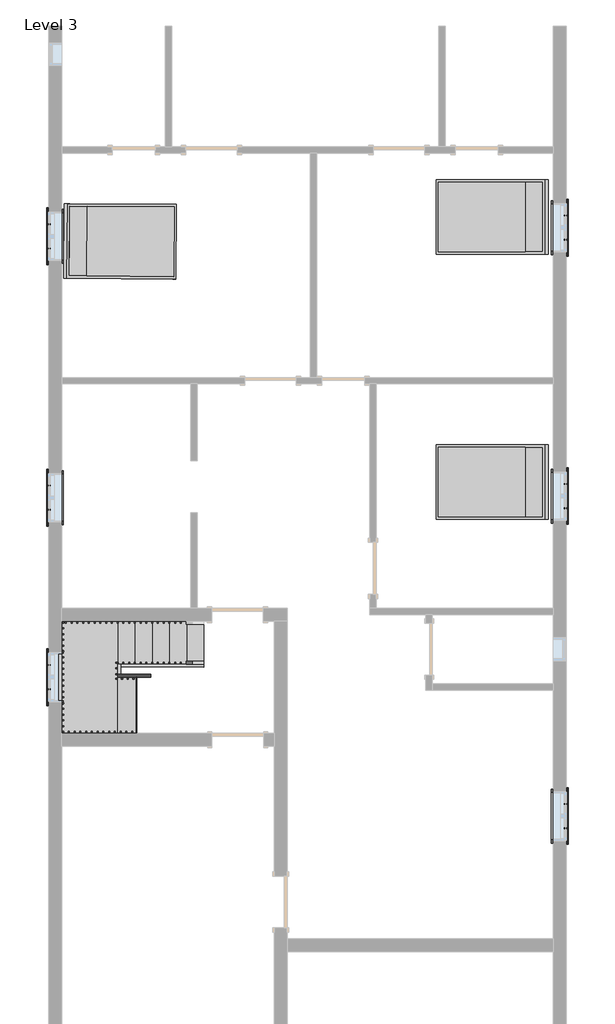
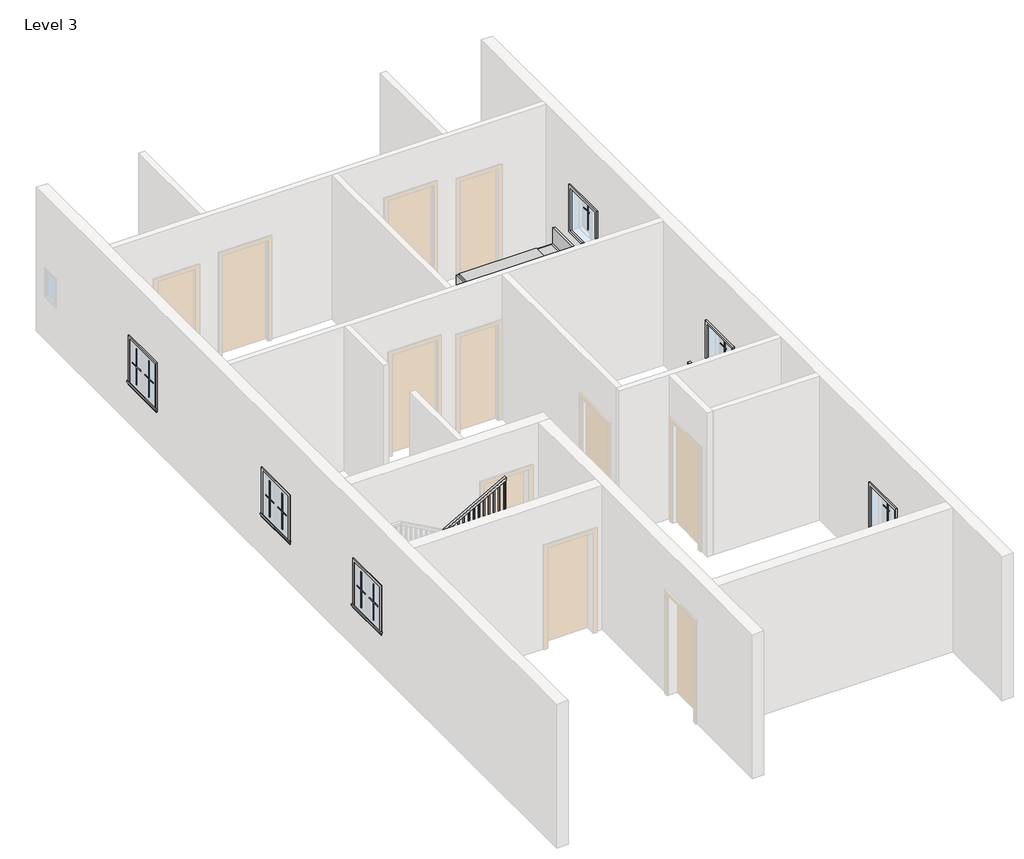
# One storey, part 3 of 3: 24 proxies, 6 members, 3 furniture elements, 1 railing, 1 stair flight.
"""IFC4 building model written with IfcOpenShell, lengths in millimetres."""

from ifc_helpers import new_model, si_unit, frame, origin, place, context, project, spatial, polyline, outline, extrude, faceted_brep, transform, mapped, element, save
from components import muntin_pattern_2x2_muntin_pattern_2x2_b3fe6957, muntin_pattern_2x2_muntin_pattern_2x2_3e0ecaf2, trim_window_exterior_flat_with_sill_41619996, trim_window_interior_flat_picture_frame_51c85655, bed_17739_bed_17739_15c61121, stair_flight_8724fc67

model = new_model("IFC4")

# Units and contexts
model_context = context("Model", 3, world=origin())
ifc_project = project(units=[si_unit("LENGTHUNIT", "METRE", prefix="MILLI")], contexts=[model_context])

# Site, building, storey
site = spatial("IfcSite", under=ifc_project)
building = spatial("IfcBuilding", under=site)
storey = spatial("IfcBuildingStorey", under=building, Name="Level 3", Elevation=3200.4)

# Proxies
placement = place(None, origin())
muntin_pattern_2x2_muntin_pattern_2x2_shape = muntin_pattern_2x2_muntin_pattern_2x2_b3fe6957(model_context)
element("IfcBuildingElementProxy", 1, Name="Muntin Pattern_2x2 : Muntin Pattern_2x2", ObjectType="Muntin Pattern_2x2 : Muntin Pattern_2x2", at=placement, inside=storey, context=model_context, shape_type="MappedRepresentation", body=[
    mapped(muntin_pattern_2x2_muntin_pattern_2x2_shape, transform((3307.2334916, 6850.4197267, 4184.65), x_axis=(0.0, -1.0, 0.0), y_axis=(1.0, 0.0, 0.0), z_axis=(0.0, 0.0, 1.0))),
])
element("IfcBuildingElementProxy", 2, Name="Muntin Pattern_2x2 : Muntin Pattern_2x2", ObjectType="Muntin Pattern_2x2 : Muntin Pattern_2x2", at=placement, inside=storey, context=model_context, shape_type="MappedRepresentation", body=[
    mapped(muntin_pattern_2x2_muntin_pattern_2x2_shape, transform((3307.2334916, 2106.9697267, 4184.65), x_axis=(0.0, -1.0, 0.0), y_axis=(1.0, 0.0, 0.0), z_axis=(0.0, 0.0, 1.0))),
])
element("IfcBuildingElementProxy", 3, Name="Muntin Pattern_2x2 : Muntin Pattern_2x2", ObjectType="Muntin Pattern_2x2 : Muntin Pattern_2x2", at=placement, inside=storey, context=model_context, shape_type="MappedRepresentation", body=[
    mapped(muntin_pattern_2x2_muntin_pattern_2x2_shape, transform((-5817.7165084, 6269.3947267, 4184.65), x_axis=(0.0, 1.0, 0.0), y_axis=(-1.0, 0.0, 0.0), z_axis=(0.0, 0.0, 1.0))),
])
element("IfcBuildingElementProxy", 4, Name="Muntin Pattern_2x2 : Muntin Pattern_2x2", ObjectType="Muntin Pattern_2x2 : Muntin Pattern_2x2", at=placement, inside=storey, context=model_context, shape_type="MappedRepresentation", body=[
    mapped(muntin_pattern_2x2_muntin_pattern_2x2_shape, transform((-5817.7165084, 1649.7697267, 4184.65), x_axis=(0.0, 1.0, 0.0), y_axis=(-1.0, 0.0, 0.0), z_axis=(0.0, 0.0, 1.0))),
])
element("IfcBuildingElementProxy", 5, Name="Muntin Pattern_2x2 : Muntin Pattern_2x2", ObjectType="Muntin Pattern_2x2 : Muntin Pattern_2x2", at=placement, inside=storey, context=model_context, shape_type="MappedRepresentation", body=[
    mapped(muntin_pattern_2x2_muntin_pattern_2x2_shape, transform((3307.2334916, -3547.7052733, 4184.65), x_axis=(0.0, -1.0, 0.0), y_axis=(1.0, 0.0, 0.0), z_axis=(0.0, 0.0, 1.0))),
])
element("IfcBuildingElementProxy", 6, Name="Muntin Pattern_2x2 : Muntin Pattern_2x2", ObjectType="Muntin Pattern_2x2 : Muntin Pattern_2x2", at=placement, inside=storey, context=model_context, shape_type="MappedRepresentation", body=[
    mapped(muntin_pattern_2x2_muntin_pattern_2x2_shape, transform((-5817.7165084, -1522.0552733, 4184.65), x_axis=(0.0, 1.0, 0.0), y_axis=(-1.0, 0.0, 0.0), z_axis=(0.0, 0.0, 1.0))),
])
muntin_pattern_2x2_muntin_pattern_2x2_2_shape = muntin_pattern_2x2_muntin_pattern_2x2_3e0ecaf2(model_context)
element("IfcBuildingElementProxy", 7, Name="Muntin Pattern_2x2 : Muntin Pattern_2x2", ObjectType="Muntin Pattern_2x2 : Muntin Pattern_2x2", at=placement, inside=storey, context=model_context, shape_type="MappedRepresentation", body=[
    mapped(muntin_pattern_2x2_muntin_pattern_2x2_2_shape, transform((3307.2334916, 6421.7947267, 4184.65), x_axis=(0.0, 1.0, 0.0), y_axis=(-1.0, 0.0, 0.0), z_axis=(0.0, 0.0, 1.0))),
])
element("IfcBuildingElementProxy", 8, Name="Muntin Pattern_2x2 : Muntin Pattern_2x2", ObjectType="Muntin Pattern_2x2 : Muntin Pattern_2x2", at=placement, inside=storey, context=model_context, shape_type="MappedRepresentation", body=[
    mapped(muntin_pattern_2x2_muntin_pattern_2x2_2_shape, transform((3307.2334916, 1678.3447267, 4184.65), x_axis=(0.0, 1.0, 0.0), y_axis=(-1.0, 0.0, 0.0), z_axis=(0.0, 0.0, 1.0))),
])
element("IfcBuildingElementProxy", 9, Name="Muntin Pattern_2x2 : Muntin Pattern_2x2", ObjectType="Muntin Pattern_2x2 : Muntin Pattern_2x2", at=placement, inside=storey, context=model_context, shape_type="MappedRepresentation", body=[
    mapped(muntin_pattern_2x2_muntin_pattern_2x2_2_shape, transform((-5817.7165084, 6698.0197267, 4184.65), x_axis=(0.0, -1.0, 0.0), y_axis=(1.0, 0.0, 0.0), z_axis=(0.0, 0.0, 1.0))),
])
element("IfcBuildingElementProxy", 10, Name="Muntin Pattern_2x2 : Muntin Pattern_2x2", ObjectType="Muntin Pattern_2x2 : Muntin Pattern_2x2", at=placement, inside=storey, context=model_context, shape_type="MappedRepresentation", body=[
    mapped(muntin_pattern_2x2_muntin_pattern_2x2_2_shape, transform((-5817.7165084, 2078.3947267, 4184.65), x_axis=(0.0, -1.0, 0.0), y_axis=(1.0, 0.0, 0.0), z_axis=(0.0, 0.0, 1.0))),
])
element("IfcBuildingElementProxy", 11, Name="Muntin Pattern_2x2 : Muntin Pattern_2x2", ObjectType="Muntin Pattern_2x2 : Muntin Pattern_2x2", at=placement, inside=storey, context=model_context, shape_type="MappedRepresentation", body=[
    mapped(muntin_pattern_2x2_muntin_pattern_2x2_2_shape, transform((3307.2334916, -3976.3302733, 4184.65), x_axis=(0.0, 1.0, 0.0), y_axis=(-1.0, 0.0, 0.0), z_axis=(0.0, 0.0, 1.0))),
])
element("IfcBuildingElementProxy", 12, Name="Muntin Pattern_2x2 : Muntin Pattern_2x2", ObjectType="Muntin Pattern_2x2 : Muntin Pattern_2x2", at=placement, inside=storey, context=model_context, shape_type="MappedRepresentation", body=[
    mapped(muntin_pattern_2x2_muntin_pattern_2x2_2_shape, transform((-5817.7165084, -1093.4302733, 4184.65), x_axis=(0.0, -1.0, 0.0), y_axis=(1.0, 0.0, 0.0), z_axis=(0.0, 0.0, 1.0))),
])
trim_window_exterior_flat_with_sill_shape = trim_window_exterior_flat_with_sill_41619996(model_context)
element("IfcBuildingElementProxy", 13, Name="Trim-Window-Exterior-Flat : with Sill", ObjectType="Trim-Window-Exterior-Flat : with Sill", at=placement, inside=storey, context=model_context, shape_type="MappedRepresentation", body=[
    mapped(trim_window_exterior_flat_with_sill_shape, transform((3316.7584916, 6636.1072267, 5029.2), x_axis=(0.0, 1.0, 0.0), y_axis=(0.0, 0.0, 1.0), z_axis=(1.0, 0.0, 0.0))),
])
element("IfcBuildingElementProxy", 14, Name="Trim-Window-Exterior-Flat : with Sill", ObjectType="Trim-Window-Exterior-Flat : with Sill", at=placement, inside=storey, context=model_context, shape_type="MappedRepresentation", body=[
    mapped(trim_window_exterior_flat_with_sill_shape, transform((3316.7584916, 1892.6572267, 5029.2), x_axis=(0.0, 1.0, 0.0), y_axis=(0.0, 0.0, 1.0), z_axis=(1.0, 0.0, 0.0))),
])
element("IfcBuildingElementProxy", 15, Name="Trim-Window-Exterior-Flat : with Sill", ObjectType="Trim-Window-Exterior-Flat : with Sill", at=placement, inside=storey, context=model_context, shape_type="MappedRepresentation", body=[
    mapped(trim_window_exterior_flat_with_sill_shape, transform((-5827.2415084, 6483.7072267, 5029.2), x_axis=(0.0, -1.0, 0.0), y_axis=(0.0, 0.0, 1.0), z_axis=(-1.0, 0.0, 0.0))),
])
element("IfcBuildingElementProxy", 16, Name="Trim-Window-Exterior-Flat : with Sill", ObjectType="Trim-Window-Exterior-Flat : with Sill", at=placement, inside=storey, context=model_context, shape_type="MappedRepresentation", body=[
    mapped(trim_window_exterior_flat_with_sill_shape, transform((-5827.2415084, 1864.0822267, 5029.2), x_axis=(0.0, -1.0, 0.0), y_axis=(0.0, 0.0, 1.0), z_axis=(-1.0, 0.0, 0.0))),
])
element("IfcBuildingElementProxy", 17, Name="Trim-Window-Exterior-Flat : with Sill", ObjectType="Trim-Window-Exterior-Flat : with Sill", at=placement, inside=storey, context=model_context, shape_type="MappedRepresentation", body=[
    mapped(trim_window_exterior_flat_with_sill_shape, transform((3316.7584916, -3762.0177733, 5029.2), x_axis=(0.0, 1.0, 0.0), y_axis=(0.0, 0.0, 1.0), z_axis=(1.0, 0.0, 0.0))),
])
element("IfcBuildingElementProxy", 18, Name="Trim-Window-Exterior-Flat : with Sill", ObjectType="Trim-Window-Exterior-Flat : with Sill", at=placement, inside=storey, context=model_context, shape_type="MappedRepresentation", body=[
    mapped(trim_window_exterior_flat_with_sill_shape, transform((-5827.2415084, -1307.7427733, 5029.2), x_axis=(0.0, -1.0, 0.0), y_axis=(0.0, 0.0, 1.0), z_axis=(-1.0, 0.0, 0.0))),
])
trim_window_interior_flat_picture_frame_shape = trim_window_interior_flat_picture_frame_51c85655(model_context)
element("IfcBuildingElementProxy", 19, Name="Trim-Window-Interior-Flat : Picture Frame", ObjectType="Trim-Window-Interior-Flat : Picture Frame", at=placement, inside=storey, context=model_context, shape_type="MappedRepresentation", body=[
    mapped(trim_window_interior_flat_picture_frame_shape, transform((3088.1584916, 6636.1072267, 5029.2), x_axis=(0.0, -1.0, 0.0), y_axis=(0.0, 0.0, 1.0), z_axis=(-1.0, 0.0, 0.0))),
])
element("IfcBuildingElementProxy", 20, Name="Trim-Window-Interior-Flat : Picture Frame", ObjectType="Trim-Window-Interior-Flat : Picture Frame", at=placement, inside=storey, context=model_context, shape_type="MappedRepresentation", body=[
    mapped(trim_window_interior_flat_picture_frame_shape, transform((3088.1584916, 1892.6572267, 5029.2), x_axis=(0.0, -1.0, 0.0), y_axis=(0.0, 0.0, 1.0), z_axis=(-1.0, 0.0, 0.0))),
])
element("IfcBuildingElementProxy", 21, Name="Trim-Window-Interior-Flat : Picture Frame", ObjectType="Trim-Window-Interior-Flat : Picture Frame", at=placement, inside=storey, context=model_context, shape_type="MappedRepresentation", body=[
    mapped(trim_window_interior_flat_picture_frame_shape, transform((-5598.6415084, 6483.7072267, 5029.2), x_axis=(0.0, 1.0, 0.0), y_axis=(0.0, 0.0, 1.0), z_axis=(1.0, 0.0, 0.0))),
])
element("IfcBuildingElementProxy", 22, Name="Trim-Window-Interior-Flat : Picture Frame", ObjectType="Trim-Window-Interior-Flat : Picture Frame", at=placement, inside=storey, context=model_context, shape_type="MappedRepresentation", body=[
    mapped(trim_window_interior_flat_picture_frame_shape, transform((-5598.6415084, 1864.0822267, 5029.2), x_axis=(0.0, 1.0, 0.0), y_axis=(0.0, 0.0, 1.0), z_axis=(1.0, 0.0, 0.0))),
])
element("IfcBuildingElementProxy", 23, Name="Trim-Window-Interior-Flat : Picture Frame", ObjectType="Trim-Window-Interior-Flat : Picture Frame", at=placement, inside=storey, context=model_context, shape_type="MappedRepresentation", body=[
    mapped(trim_window_interior_flat_picture_frame_shape, transform((3088.1584916, -3762.0177733, 5029.2), x_axis=(0.0, -1.0, 0.0), y_axis=(0.0, 0.0, 1.0), z_axis=(-1.0, 0.0, 0.0))),
])
element("IfcBuildingElementProxy", 24, Name="Trim-Window-Interior-Flat : Picture Frame", ObjectType="Trim-Window-Interior-Flat : Picture Frame", at=placement, inside=storey, context=model_context, shape_type="MappedRepresentation", body=[
    mapped(trim_window_interior_flat_picture_frame_shape, transform((-5598.6415084, -1307.7427733, 5029.2), x_axis=(0.0, 1.0, 0.0), y_axis=(0.0, 0.0, 1.0), z_axis=(1.0, 0.0, 0.0))),
])

# Furniture
bed_17739_bed_17739_shape = bed_17739_bed_17739_15c61121(model_context)
element("IfcFurniture", 25, ObjectType="Bed_17739 : Bed_17739", at=placement, inside=storey, context=model_context, shape_type="MappedRepresentation", body=[
    mapped(bed_17739_bed_17739_shape, transform((-4543.6279345, 6394.2844586, 3200.4), x_axis=(0.007593038844487308, 0.9999711724650396, 0.0), y_axis=(-0.9999711724650396, 0.007593038844487308, 0.0), z_axis=(0.0, 0.0, 1.0))),
])
element("IfcFurniture", 26, ObjectType="Bed_17739 : Bed_17739", at=placement, inside=storey, context=model_context, shape_type="MappedRepresentation", body=[
    mapped(bed_17739_bed_17739_shape, transform((1983.2584916, 6826.6072267, 3200.4), x_axis=(0.0, -1.0, 0.0), y_axis=(1.0, 0.0, 0.0), z_axis=(0.0, 0.0, 1.0))),
])
element("IfcFurniture", 27, ObjectType="Bed_17739 : Bed_17739", at=placement, inside=storey, context=model_context, shape_type="MappedRepresentation", body=[
    mapped(bed_17739_bed_17739_shape, transform((1983.2584916, 2140.3072267, 3200.4), x_axis=(0.0, -1.0, 0.0), y_axis=(1.0, 0.0, 0.0), z_axis=(0.0, 0.0, 1.0))),
])

# Members
element("IfcMember", 28, ObjectType="Stringer - 2\" Width", at=placement, inside=storey, context=model_context, shape_type="SweptSolid", body=[
    extrude(outline(polyline([(3200.4, -3084.0415084), (3407.9983948, -3084.0415084), (4226.4428392, -4557.2415084), (3877.7641651, -4557.2415084), (3200.4, -3337.9860112), (3200.4, -3084.0415084)])), frame((0.0, -1127.4758739, 0.0), z_axis=(0.0, 1.0, 0.0), x_axis=(0.0, 0.0, 1.0)), (0.0, 0.0, 1.0), 50.8),
])
element("IfcMember", 29, ObjectType="Stringer - 2\" Width", at=placement, inside=storey, context=model_context, shape_type="SweptSolid", body=[
    extrude(outline(polyline([(-4608.0415084, -1076.6758739), (-4557.2415084, -1076.6758739), (-4557.2415084, -1256.9427733), (-4608.0415084, -1256.9427733), (-4608.0415084, -1076.6758739)])), frame((0.0, 0.0, 3987.8), z_axis=(0.0, 0.0, 1.0), x_axis=(1.0, 0.0, 0.0)), (0.0, 0.0, 1.0), 304.8),
])
element("IfcMember", 30, ObjectType="Stringer - 2\" Width", at=placement, inside=storey, context=model_context, shape_type="SweptSolid", body=[
    extrude(outline(polyline([(4423.9983948, -4608.0415084), (4075.3197207, -4608.0415084), (4921.9863873, -3084.0415084), (5270.6650614, -3084.0415084), (4423.9983948, -4608.0415084)])), frame((0.0, -1307.7427733, 0.0), z_axis=(0.0, 1.0, 0.0), x_axis=(0.0, 0.0, 1.0)), (0.0, 0.0, 1.0), 50.8),
])
element("IfcMember", 31, ObjectType="Stringer - 2\" Width", at=placement, inside=storey, context=model_context, shape_type="SweptSolid", body=[
    extrude(outline(polyline([(3200.4, -3084.0415084), (3407.9983948, -3084.0415084), (4292.6, -4676.3243978), (4292.6, -5303.9460112), (3200.4, -3337.9860112), (3200.4, -3084.0415084)])), frame((0.0, -317.1427733, 0.0), z_axis=(0.0, 1.0, 0.0), x_axis=(0.0, 0.0, 1.0)), (0.0, 0.0, 1.0), 50.8),
])
element("IfcMember", 32, ObjectType="Stringer - 2\" Width", at=placement, inside=storey, context=model_context, shape_type="SweptSolid", body=[
    extrude(outline(polyline([(-5649.4415084, -266.3427733), (-5598.6415084, -266.3427733), (-5598.6415084, -2298.3427733), (-5649.4415084, -2298.3427733), (-5649.4415084, -266.3427733)])), frame((0.0, 0.0, 3987.8), z_axis=(0.0, 0.0, 1.0), x_axis=(1.0, 0.0, 0.0)), (0.0, 0.0, 1.0), 304.8),
])
element("IfcMember", 33, ObjectType="Stringer - 2\" Width", at=placement, inside=storey, context=model_context, shape_type="SweptSolid", body=[
    extrude(outline(polyline([(3987.8, -4765.5770056), (4921.9863873, -3084.0415084), (5270.6650614, -3084.0415084), (3987.8, -5393.198619), (3987.8, -4765.5770056)])), frame((0.0, -2349.1427733, 0.0), z_axis=(0.0, 1.0, 0.0), x_axis=(0.0, 0.0, 1.0)), (0.0, 0.0, 1.0), 50.8),
])

# Railing
element("IfcRailing", 34, ObjectType="Handrail - Rectangular", at=placement, inside=storey, context=model_context, shape_type="SolidModel", body=[
    faceted_brep([(-3084.0415084, -1076.6758739, 4284.1333333), (-3084.0415084, -1076.6758739, 4226.020221), (-3084.0415084, -1025.8758739, 4226.020221), (-3084.0415084, -1025.8758739, 4284.1333333), (-4531.8415084, -1076.6758739, 5088.4666667), (-4582.6415084, -1076.6758739, 5058.5757765), (-4582.6415084, -1025.8758739, 5058.5757765), (-4531.8415084, -1025.8758739, 5088.4666667), (-4531.8415084, -1076.6758739, 5130.8), (-4582.6415084, -1076.6758739, 5080.0), (-4582.6415084, -1025.8758739, 5080.0), (-4531.8415084, -1025.8758739, 5130.8), (-4608.0415084, -1076.6758739, 5130.8), (-4608.0415084, -1076.6758739, 5080.0), (-4658.8415084, -1025.8758739, 5080.0), (-4658.8415084, -1025.8758739, 5130.8), (-4608.0415084, -1152.8758739, 5130.8), (-4608.0415084, -1152.8758739, 5080.0), (-4658.8415084, -1152.8758739, 5080.0), (-4658.8415084, -1152.8758739, 5130.8), (-4608.0415084, -1231.5427733, 5130.8), (-4608.0415084, -1282.3427733, 5080.0), (-4658.8415084, -1282.3427733, 5080.0), (-4658.8415084, -1231.5427733, 5130.8), (-4608.0415084, -1231.5427733, 5342.4666667), (-4608.0415084, -1282.3427733, 5291.6666667), (-4658.8415084, -1282.3427733, 5291.6666667), (-4658.8415084, -1231.5427733, 5342.4666667), (-4608.0415084, -1307.7427733, 5342.4666667), (-4608.0415084, -1307.7427733, 5291.6666667), (-4658.8415084, -1358.5427733, 5291.6666667), (-4658.8415084, -1358.5427733, 5342.4666667), (-4531.8415084, -1307.7427733, 5342.4666667), (-4518.6779062, -1307.7427733, 5291.6666667), (-4518.6779062, -1358.5427733, 5291.6666667), (-4531.8415084, -1358.5427733, 5342.4666667), (-3084.0415084, -1307.7427733, 6146.8), (-3084.0415084, -1358.5427733, 6146.8), (-3084.0415084, -1358.5427733, 6088.6868876), (-3084.0415084, -1307.7427733, 6088.6868876)], [[[0, 1, 2, 3]], [[1, 0, 4, 5]], [[2, 1, 5, 6]], [[3, 2, 6, 7]], [[0, 3, 7, 4]], [[5, 4, 8, 9]], [[6, 5, 9, 10]], [[7, 6, 10, 11]], [[4, 7, 11, 8]], [[9, 8, 12, 13]], [[10, 9, 13, 14]], [[11, 10, 14, 15]], [[8, 11, 15, 12]], [[13, 12, 16, 17]], [[14, 13, 17, 18]], [[15, 14, 18, 19]], [[12, 15, 19, 16]], [[17, 16, 20, 21]], [[18, 17, 21, 22]], [[19, 18, 22, 23]], [[16, 19, 23, 20]], [[21, 20, 24, 25]], [[22, 21, 25, 26]], [[23, 22, 26, 27]], [[20, 23, 27, 24]], [[25, 24, 28, 29]], [[26, 25, 29, 30]], [[27, 26, 30, 31]], [[24, 27, 31, 28]], [[29, 28, 32, 33]], [[30, 29, 33, 34]], [[31, 30, 34, 35]], [[28, 31, 35, 32]], [[36, 37, 38, 39]], [[33, 32, 36, 39]], [[34, 33, 39, 38]], [[35, 34, 38, 37]], [[32, 35, 37, 36]]]),
    extrude(outline(polyline([(6069.2841099, -3118.9665084), (5063.0666667, -3118.9665084), (5063.0666667, -3099.9165084), (6079.8674432, -3099.9165084), (6069.2841099, -3118.9665084)])), frame((0.0, -1342.6677733, 0.0), z_axis=(0.0, 1.0, 0.0), x_axis=(0.0, 0.0, 1.0)), (0.0, 0.0, 1.0), 19.05),
    extrude(outline(polyline([(6012.8396654, -3220.5665084), (5063.0666667, -3220.5665084), (5063.0666667, -3201.5165084), (6023.4229988, -3201.5165084), (6012.8396654, -3220.5665084)])), frame((0.0, -1342.6677733, 0.0), z_axis=(0.0, 1.0, 0.0), x_axis=(0.0, 0.0, 1.0)), (0.0, 0.0, 1.0), 19.05),
    extrude(outline(polyline([(5956.395221, -3322.1665084), (5063.0666667, -3322.1665084), (5063.0666667, -3303.1165084), (5966.9785543, -3303.1165084), (5956.395221, -3322.1665084)])), frame((0.0, -1342.6677733, 0.0), z_axis=(0.0, 1.0, 0.0), x_axis=(0.0, 0.0, 1.0)), (0.0, 0.0, 1.0), 19.05),
    extrude(outline(polyline([(5899.9507765, -3423.7665084), (4893.7333333, -3423.7665084), (4893.7333333, -3404.7165084), (5910.5341099, -3404.7165084), (5899.9507765, -3423.7665084)])), frame((0.0, -1342.6677733, 0.0), z_axis=(0.0, 1.0, 0.0), x_axis=(0.0, 0.0, 1.0)), (0.0, 0.0, 1.0), 19.05),
    extrude(outline(polyline([(5843.5063321, -3525.3665084), (4893.7333333, -3525.3665084), (4893.7333333, -3506.3165084), (5854.0896654, -3506.3165084), (5843.5063321, -3525.3665084)])), frame((0.0, -1342.6677733, 0.0), z_axis=(0.0, 1.0, 0.0), x_axis=(0.0, 0.0, 1.0)), (0.0, 0.0, 1.0), 19.05),
    extrude(outline(polyline([(5787.0618876, -3626.9665084), (4893.7333333, -3626.9665084), (4893.7333333, -3607.9165084), (5797.645221, -3607.9165084), (5787.0618876, -3626.9665084)])), frame((0.0, -1342.6677733, 0.0), z_axis=(0.0, 1.0, 0.0), x_axis=(0.0, 0.0, 1.0)), (0.0, 0.0, 1.0), 19.05),
    extrude(outline(polyline([(5730.6174432, -3728.5665084), (4724.4, -3728.5665084), (4724.4, -3709.5165084), (5741.2007765, -3709.5165084), (5730.6174432, -3728.5665084)])), frame((0.0, -1342.6677733, 0.0), z_axis=(0.0, 1.0, 0.0), x_axis=(0.0, 0.0, 1.0)), (0.0, 0.0, 1.0), 19.05),
    extrude(outline(polyline([(5674.1729988, -3830.1665084), (4724.4, -3830.1665084), (4724.4, -3811.1165084), (5684.7563321, -3811.1165084), (5674.1729988, -3830.1665084)])), frame((0.0, -1342.6677733, 0.0), z_axis=(0.0, 1.0, 0.0), x_axis=(0.0, 0.0, 1.0)), (0.0, 0.0, 1.0), 19.05),
    extrude(outline(polyline([(5617.7285543, -3931.7665084), (4724.4, -3931.7665084), (4724.4, -3912.7165084), (5628.3118876, -3912.7165084), (5617.7285543, -3931.7665084)])), frame((0.0, -1342.6677733, 0.0), z_axis=(0.0, 1.0, 0.0), x_axis=(0.0, 0.0, 1.0)), (0.0, 0.0, 1.0), 19.05),
    extrude(outline(polyline([(5561.2841099, -4033.3665084), (4555.0666667, -4033.3665084), (4555.0666667, -4014.3165084), (5571.8674432, -4014.3165084), (5561.2841099, -4033.3665084)])), frame((0.0, -1342.6677733, 0.0), z_axis=(0.0, 1.0, 0.0), x_axis=(0.0, 0.0, 1.0)), (0.0, 0.0, 1.0), 19.05),
    extrude(outline(polyline([(5504.8396654, -4134.9665084), (4555.0666667, -4134.9665084), (4555.0666667, -4115.9165084), (5515.4229988, -4115.9165084), (5504.8396654, -4134.9665084)])), frame((0.0, -1342.6677733, 0.0), z_axis=(0.0, 1.0, 0.0), x_axis=(0.0, 0.0, 1.0)), (0.0, 0.0, 1.0), 19.05),
    extrude(outline(polyline([(5448.395221, -4236.5665084), (4555.0666667, -4236.5665084), (4555.0666667, -4217.5165084), (5458.9785543, -4217.5165084), (5448.395221, -4236.5665084)])), frame((0.0, -1342.6677733, 0.0), z_axis=(0.0, 1.0, 0.0), x_axis=(0.0, 0.0, 1.0)), (0.0, 0.0, 1.0), 19.05),
    extrude(outline(polyline([(5391.9507765, -4338.1665084), (4385.7333333, -4338.1665084), (4385.7333333, -4319.1165084), (5402.5341099, -4319.1165084), (5391.9507765, -4338.1665084)])), frame((0.0, -1342.6677733, 0.0), z_axis=(0.0, 1.0, 0.0), x_axis=(0.0, 0.0, 1.0)), (0.0, 0.0, 1.0), 19.05),
    extrude(outline(polyline([(5335.5063321, -4439.7665084), (4385.7333333, -4439.7665084), (4385.7333333, -4420.7165084), (5346.0896654, -4420.7165084), (5335.5063321, -4439.7665084)])), frame((0.0, -1342.6677733, 0.0), z_axis=(0.0, 1.0, 0.0), x_axis=(0.0, 0.0, 1.0)), (0.0, 0.0, 1.0), 19.05),
    extrude(outline(polyline([(5279.0618876, -4541.3665084), (4385.7333333, -4541.3665084), (4385.7333333, -4522.3165084), (5289.645221, -4522.3165084), (5279.0618876, -4541.3665084)])), frame((0.0, -1342.6677733, 0.0), z_axis=(0.0, 1.0, 0.0), x_axis=(0.0, 0.0, 1.0)), (0.0, 0.0, 1.0), 19.05),
    extrude(outline(polyline([(-4623.9165084, -1244.9508739), (-4623.9165084, -1264.0008739), (-4642.9665084, -1264.0008739), (-4642.9665084, -1244.9508739), (-4623.9165084, -1244.9508739)])), frame((0.0, 0.0, 4216.4), z_axis=(0.0, 0.0, 1.0), x_axis=(1.0, 0.0, 0.0)), (0.0, 0.0, 1.0), 1075.2666667),
    extrude(outline(polyline([(-4623.9165084, -1143.3508739), (-4623.9165084, -1162.4008739), (-4642.9665084, -1162.4008739), (-4642.9665084, -1143.3508739), (-4623.9165084, -1143.3508739)])), frame((0.0, 0.0, 4216.4), z_axis=(0.0, 0.0, 1.0), x_axis=(1.0, 0.0, 0.0)), (0.0, 0.0, 1.0), 863.6),
    extrude(outline(polyline([(-4598.5165084, -1060.8008739), (-4617.5665084, -1060.8008739), (-4617.5665084, -1041.7508739), (-4598.5165084, -1041.7508739), (-4598.5165084, -1060.8008739)])), frame((0.0, 0.0, 4216.4), z_axis=(0.0, 0.0, 1.0), x_axis=(1.0, 0.0, 0.0)), (0.0, 0.0, 1.0), 863.6),
    extrude(outline(polyline([(5021.5341099, -4515.9665084), (4047.0666667, -4515.9665084), (4047.0666667, -4496.9165084), (5010.9507765, -4496.9165084), (5021.5341099, -4515.9665084)])), frame((0.0, -1060.8008739, 0.0), z_axis=(0.0, 1.0, 0.0), x_axis=(0.0, 0.0, 1.0)), (0.0, 0.0, 1.0), 19.05),
    extrude(outline(polyline([(4965.0896654, -4414.3665084), (4047.0666667, -4414.3665084), (4047.0666667, -4395.3165084), (4954.5063321, -4395.3165084), (4965.0896654, -4414.3665084)])), frame((0.0, -1060.8008739, 0.0), z_axis=(0.0, 1.0, 0.0), x_axis=(0.0, 0.0, 1.0)), (0.0, 0.0, 1.0), 19.05),
    extrude(outline(polyline([(4908.645221, -4312.7665084), (4047.0666667, -4312.7665084), (4047.0666667, -4293.7165084), (4898.0618876, -4293.7165084), (4908.645221, -4312.7665084)])), frame((0.0, -1060.8008739, 0.0), z_axis=(0.0, 1.0, 0.0), x_axis=(0.0, 0.0, 1.0)), (0.0, 0.0, 1.0), 19.05),
    extrude(outline(polyline([(4852.2007765, -4211.1665084), (3877.7333333, -4211.1665084), (3877.7333333, -4192.1165084), (4841.6174432, -4192.1165084), (4852.2007765, -4211.1665084)])), frame((0.0, -1060.8008739, 0.0), z_axis=(0.0, 1.0, 0.0), x_axis=(0.0, 0.0, 1.0)), (0.0, 0.0, 1.0), 19.05),
    extrude(outline(polyline([(4795.7563321, -4109.5665084), (3877.7333333, -4109.5665084), (3877.7333333, -4090.5165084), (4785.1729988, -4090.5165084), (4795.7563321, -4109.5665084)])), frame((0.0, -1060.8008739, 0.0), z_axis=(0.0, 1.0, 0.0), x_axis=(0.0, 0.0, 1.0)), (0.0, 0.0, 1.0), 19.05),
    extrude(outline(polyline([(4739.3118876, -4007.9665084), (3877.7333333, -4007.9665084), (3877.7333333, -3988.9165084), (4728.7285543, -3988.9165084), (4739.3118876, -4007.9665084)])), frame((0.0, -1060.8008739, 0.0), z_axis=(0.0, 1.0, 0.0), x_axis=(0.0, 0.0, 1.0)), (0.0, 0.0, 1.0), 19.05),
    extrude(outline(polyline([(4682.8674432, -3906.3665084), (3708.4, -3906.3665084), (3708.4, -3887.3165084), (4672.2841099, -3887.3165084), (4682.8674432, -3906.3665084)])), frame((0.0, -1060.8008739, 0.0), z_axis=(0.0, 1.0, 0.0), x_axis=(0.0, 0.0, 1.0)), (0.0, 0.0, 1.0), 19.05),
    extrude(outline(polyline([(4626.4229988, -3804.7665084), (3708.4, -3804.7665084), (3708.4, -3785.7165084), (4615.8396654, -3785.7165084), (4626.4229988, -3804.7665084)])), frame((0.0, -1060.8008739, 0.0), z_axis=(0.0, 1.0, 0.0), x_axis=(0.0, 0.0, 1.0)), (0.0, 0.0, 1.0), 19.05),
    extrude(outline(polyline([(4569.9785543, -3703.1665084), (3708.4, -3703.1665084), (3708.4, -3684.1165084), (4559.395221, -3684.1165084), (4569.9785543, -3703.1665084)])), frame((0.0, -1060.8008739, 0.0), z_axis=(0.0, 1.0, 0.0), x_axis=(0.0, 0.0, 1.0)), (0.0, 0.0, 1.0), 19.05),
    extrude(outline(polyline([(4513.5341099, -3601.5665084), (3539.0666667, -3601.5665084), (3539.0666667, -3582.5165084), (4502.9507765, -3582.5165084), (4513.5341099, -3601.5665084)])), frame((0.0, -1060.8008739, 0.0), z_axis=(0.0, 1.0, 0.0), x_axis=(0.0, 0.0, 1.0)), (0.0, 0.0, 1.0), 19.05),
    extrude(outline(polyline([(4457.0896654, -3499.9665084), (3539.0666667, -3499.9665084), (3539.0666667, -3480.9165084), (4446.5063321, -3480.9165084), (4457.0896654, -3499.9665084)])), frame((0.0, -1060.8008739, 0.0), z_axis=(0.0, 1.0, 0.0), x_axis=(0.0, 0.0, 1.0)), (0.0, 0.0, 1.0), 19.05),
    extrude(outline(polyline([(4400.645221, -3398.3665084), (3539.0666667, -3398.3665084), (3539.0666667, -3379.3165084), (4390.0618876, -3379.3165084), (4400.645221, -3398.3665084)])), frame((0.0, -1060.8008739, 0.0), z_axis=(0.0, 1.0, 0.0), x_axis=(0.0, 0.0, 1.0)), (0.0, 0.0, 1.0), 19.05),
    extrude(outline(polyline([(4344.2007765, -3296.7665084), (3369.7333333, -3296.7665084), (3369.7333333, -3277.7165084), (4333.6174432, -3277.7165084), (4344.2007765, -3296.7665084)])), frame((0.0, -1060.8008739, 0.0), z_axis=(0.0, 1.0, 0.0), x_axis=(0.0, 0.0, 1.0)), (0.0, 0.0, 1.0), 19.05),
    extrude(outline(polyline([(4287.7563321, -3195.1665084), (3369.7333333, -3195.1665084), (3369.7333333, -3176.1165084), (4277.1729988, -3176.1165084), (4287.7563321, -3195.1665084)])), frame((0.0, -1060.8008739, 0.0), z_axis=(0.0, 1.0, 0.0), x_axis=(0.0, 0.0, 1.0)), (0.0, 0.0, 1.0), 19.05),
    extrude(outline(polyline([(-4623.9165084, -1323.6177733), (-4623.9165084, -1342.6677733), (-4642.9665084, -1342.6677733), (-4642.9665084, -1323.6177733), (-4623.9165084, -1323.6177733)])), frame((0.0, 0.0, 4216.4), z_axis=(0.0, 0.0, 1.0), x_axis=(1.0, 0.0, 0.0)), (0.0, 0.0, 1.0), 1075.2666667),
    extrude(outline(polyline([(-4623.9165084, -1060.8008739), (-4642.9665084, -1060.8008739), (-4642.9665084, -1041.7508739), (-4623.9165084, -1041.7508739), (-4623.9165084, -1060.8008739)])), frame((0.0, 0.0, 4216.4), z_axis=(0.0, 0.0, 1.0), x_axis=(1.0, 0.0, 0.0)), (0.0, 0.0, 1.0), 863.6),
    extrude(outline(polyline([(6078.1035543, -3103.0915084), (5063.0666667, -3103.0915084), (5063.0666667, -3084.0415084), (6088.6868876, -3084.0415084), (6078.1035543, -3103.0915084)])), frame((0.0, -1342.6677733, 0.0), z_axis=(0.0, 1.0, 0.0), x_axis=(0.0, 0.0, 1.0)), (0.0, 0.0, 1.0), 19.05),
    extrude(outline(polyline([(4236.6035543, -3103.0915084), (3369.7333333, -3103.0915084), (3369.7333333, -3084.0415084), (4226.020221, -3084.0415084), (4236.6035543, -3103.0915084)])), frame((0.0, -1060.8008739, 0.0), z_axis=(0.0, 1.0, 0.0), x_axis=(0.0, 0.0, 1.0)), (0.0, 0.0, 1.0), 19.05),
])

# Stair flight
stair_flight_shape = stair_flight_8724fc67(model_context)
element("IfcStairFlight", 35, ObjectType="2\" Tread 1\" Nosing 1/4\" Riser", at=placement, inside=storey, context=model_context, shape_type="MappedRepresentation", body=[
    mapped(stair_flight_shape, transform((0.0, 0.0, 0.0), x_axis=(1.0, 0.0, 0.0), y_axis=(0.0, 1.0, 0.0), z_axis=(0.0, 0.0, 1.0))),
])

save(model, "model.ifc")

# Revit data of these elements
# Type "Muntin Pattern_2x2 : Muntin Pattern_2x2"
#   Width [instance default] = 4' - 0"
#   Thickness = 0' - 0 1/2"
#   Height [instance default] = 4' - 0"
#   Distance = 0' - 0 3/4"
#   Interior Material [instance default] = none
#   Exterior Material [instance default] = none
#   Default Elevation = 0
# Type "Trim-Window-Exterior-Flat : with Sill"
#   Trim Width = 0' - 2 1/4"
#   Trim Thickness_Picture Frame = 0' - 1 1/4"
#   Trim Thickness_with Sill = 0' - 0 3/4"
#   Sill Thickness = 0' - 1 1/4"
#   Opening Width [instance default] = 2' - 0"
#   Opening Height [instance default] = 3' - 0"
#   Default Elevation = 4' - 0"
#   Sill = yes
#   Picture Frame = no
#   Trim Material [instance default] = none
# Type "Trim-Window-Interior-Flat : Picture Frame"
#   Trim Thickness_Picture Frame = 0' - 1 1/4"
#   Trim Width = 0' - 2 1/4"
#   Trim Thickness_with Sill = 0' - 0 3/4"
#   Sill Thickness = 0' - 1 1/4"
#   Opening Width [instance default] = 2' - 0"
#   Opening Height [instance default] = 3' - 0"
#   Default Elevation = 4' - 0"
#   Sill = no
#   Picture Frame = yes
#   Trim Material [instance default] = none
# Type "Bed_17739 : Bed_17739"
#   Default Elevation = 0
# Type "Handrail - Rectangular"
#   Assembly Code = "C2010400"
#   built-in parameter 1008612 = 0.0416667 (stored number, unit not read)
#   built-in parameter 1008611 = 0.0416667 (stored number, unit not read)
#   built-in parameter 1008609 = 0.333333 (stored number, unit not read)
#   built-in parameter 1008604 = 0.166667 (stored number, unit not read)
#   built-in parameter 1008603 = 0.166667 (stored number, unit not read)
#   Railing Height = 3' - 0"
#   built-in parameter 1008630 = 2
#   built-in parameter 1008610 = 2
#   built-in parameter 1008618 = Baluster - Square : 3/4"
# Elements 1, 2, 3, 4, 5, 6, 7, 8, 9, 10, 11, 12 (IfcBuildingElementProxy, "Muntin Pattern_2x2 : Muntin Pattern_2x2")
#   Width = 0' - 11 5/8"
#   Height = 2' - 6 1/2"
#   Interior Material = Wood - Stained
#   Exterior Material = Clad - White
#   Phase Created = New Construction
#   Materials on its faces: "Clad - White", "Wood - Stained"
# Elements 13, 14, 15, 16, 17, 18 (IfcBuildingElementProxy, "Trim-Window-Exterior-Flat : with Sill")
#   Opening Width = 2' - 10"
#   Opening Height = 3' - 0"
#   Trim Material = Clad - White
#   Phase Created = New Construction
#   Materials on its faces: "Clad - White"
# Elements 19, 20, 21, 22, 23, 24 (IfcBuildingElementProxy, "Trim-Window-Interior-Flat : Picture Frame")
#   Opening Width = 2' - 10"
#   Opening Height = 3' - 0"
#   Trim Material = Wood - Stained
#   Phase Created = New Construction
#   Materials on its faces: "Wood - Stained"
# Elements 25, 26, 27 (IfcFurniture, "Bed_17739 : Bed_17739")
#   Phase Created = New Construction
#   Materials on its faces: "legs", "sheets", "bed frame", "Blanket"
# Elements 28, 29, 30, 31, 32, 33 (IfcMember, "Stringer - 2\" Width")
#   Phase Created = New Construction
# Element 34 (IfcRailing, "Handrail - Rectangular")
#   Phase Created = New Construction
# Element 35 (IfcStairFlight, "2\" Tread 1\" Nosing 1/4\" Riser")
#   Phase Created = New Construction
# Materials
#   "Clad - White": class "Wood", colour RGB 242 242 238, transparency 0, Cost = 0
#   "Wood - Stained": class "Wood", colour RGB 224 178 126, transparency 0, Cost = 0
#   "legs": colour RGB 90 73 37, transparency 0, Cost = 0
#   "sheets": colour RGB 200 195 176, transparency 0, Cost = 0
#   "bed frame": colour RGB 90 73 37, transparency 0, Cost = 0
#   "Blanket": class "System", colour RGB 59 0 1, transparency 0, Cost = 0
